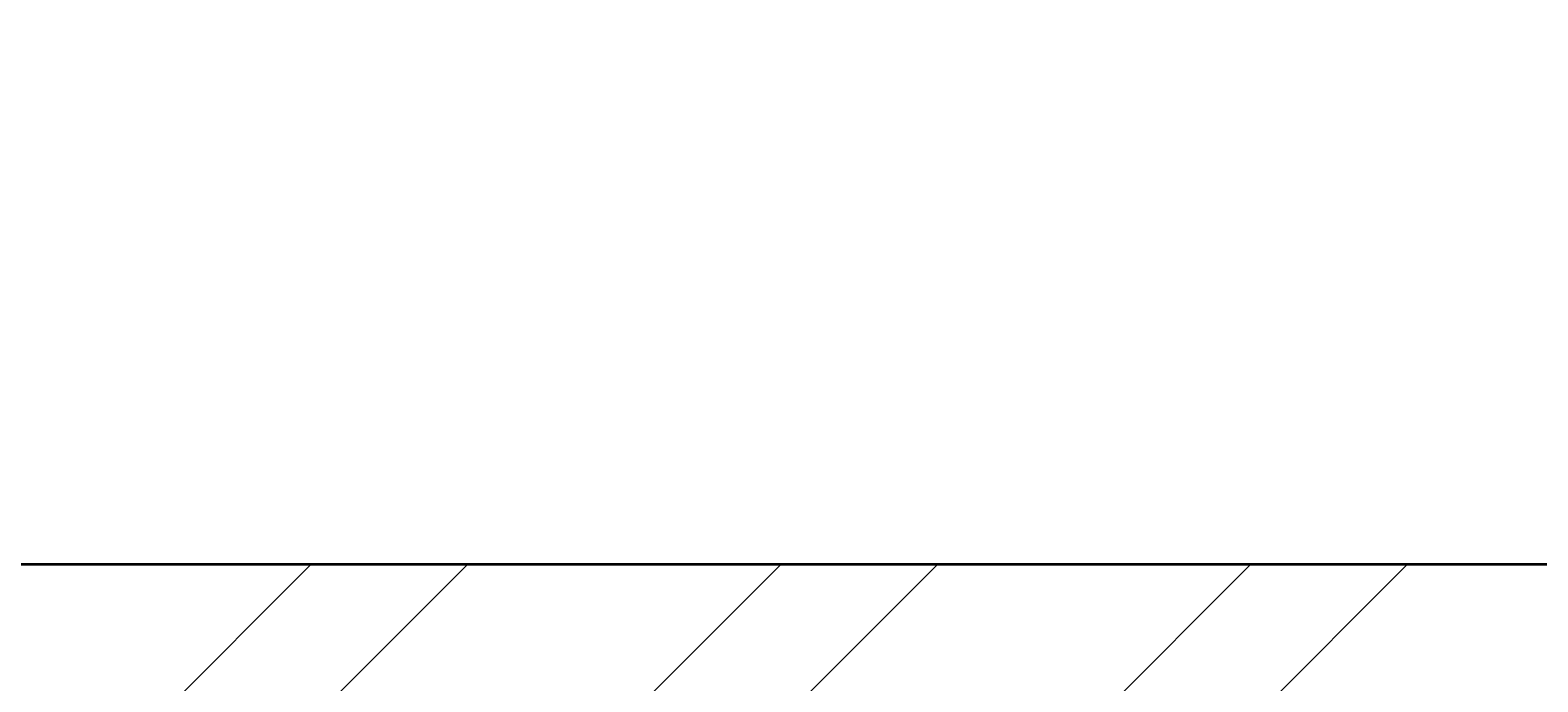
# Model space of a CAD drawing. Units: inches. Extents: x 1962 to 2771, y 1245 to 2660.
# Tile 51 of 114: x 2160 to 2204, y 2030 to 2049. Entities that reach past the tile are written whole.
import ezdxf

# ---------------------------------------------------------------- set-up
doc = ezdxf.new("R2010")
doc.units = ezdxf.units.IN
for name, color, linetype, lineweight in [('A-ANNO-DIMS', 2, 'Continuous', 18), ('A-WALL', 7, 'Continuous', 35), ('A-WALL-PATT', 252, 'Continuous', 13)]:
    doc.layers.add(name, color=color, linetype=linetype, lineweight=lineweight)
doc.styles.get("Standard").update_dxf_attribs({"font": 'arial.ttf'})
doc.dimstyles.get("Standard").update_dxf_attribs({"dimtxt": 0.18, "dimasz": 0.18, "dimexe": 0.18, "dimexo": 0.0625, "dimgap": 0.09, "dimtad": 0, "dimtih": 1, "dimtoh": 1, "dimdec": 4, "dimzin": 0, "dimdsep": 46, "dimtxsty": 'Standard', "dimcen": 0.09, "dimadec": 0, "dimazin": 0, "dimtfac": 1, "dimtdec": 4, "dimtofl": 0, "dimtmove": 0, "dimatfit": 3, "dimfxl": 1, "dimtolj": 1, "dimtzin": 0, "dimarcsym": 0})

# ---------------------------------------------------------------- blocks, each defined once
blk = doc.blocks.new('*D40')
at = {"layer": 'A-ANNO-DIMS', "color": 0, "lineweight": -2, "transparency": 16777216}
for p, q in [((2072.02, 2033.906), (2072.02, 2583.474)), ((2072.2, 2583.294), (2366.02, 2583.294)), ((2660.627, 2583.294), (2366.808, 2583.294)), ((2660.807, 2524.406), (2660.807, 2583.474))]:
    blk.add_line(p, q, dxfattribs=at)
at = {"layer": 'A-ANNO-DIMS', "color": 0, "transparency": 16777216}
for points in [[(2072.2, 2583.324), (2072.2, 2583.264), (2072.02, 2583.294)], [(2660.627, 2583.324), (2660.627, 2583.264), (2660.807, 2583.294)]]:
    blk.add_solid(points, dxfattribs=at)
at = {"layer": 'Defpoints', "color": 0, "transparency": 16777216}
for p in [(2660.807, 2583.294), (2660.807, 2524.344), (2072.02, 2033.844)]:
    blk.add_point(p, dxfattribs=at)
at = {"layer": 'A-ANNO-DIMS', "color": 0, "transparency": 16777216, "insert": (2366.414, 2583.294), "char_height": 0.18, "attachment_point": 5}
blk.add_mtext('\\A1;588.8', dxfattribs=at)

msp = doc.modelspace()

# ---------------------------------------------------------------- hatches: boundary and pattern name
at = {"layer": 'A-WALL-PATT'}
h = msp.add_hatch(dxfattribs=at)
h.set_pattern_fill('ANSI32', color=256)
h.paths.add_polyline_path([(2090.8074, 2467.3437), (2141.6481, 2467.3437), (2141.6481, 2469.5937), (2141.6481, 2471.8437), (2086.3074, 2471.8437), (2086.3074, 2422.5333), (2090.8074, 2422.5333)])
h.paths.add_polyline_path([(2282.7664, 2471.8437), (2204.8982, 2471.8437), (2204.8982, 2467.3437), (2234.8074, 2467.3437), (2234.8074, 2311.3437), (2228.7492, 2311.3437), (2228.7492, 2306.8437), (2234.8074, 2306.8437), (2331.9227, 2306.8437), (2331.9227, 2309.0937), (2331.9227, 2311.3437), (2239.3074, 2311.3437), (2239.3074, 2467.3437), (2282.7664, 2467.3437), (2282.7664, 2469.5937)])
h.paths.add_polyline_path([(2471.4531, 2519.8437), (2552.011, 2519.8437), (2564.3996, 2519.8437), (2564.3996, 2511.1389), (2568.8996, 2511.1389), (2568.8996, 2524.3437), (2466.9531, 2524.3437), (2466.9531, 2471.8437), (2450.0749, 2471.8437), (2446.4672, 2471.8437), (2446.4672, 2467.3437), (2450.0749, 2467.3437), (2475.9988, 2467.3437), (2475.9988, 2469.5937), (2475.9988, 2471.8437), (2471.4531, 2471.8437)])
h.paths.add_polyline_path([(2575.2231, 2469.5937), (2575.2231, 2471.8437), (2568.8996, 2471.8437), (2568.8996, 2487.1389), (2564.3996, 2487.1389), (2564.3996, 2471.8437), (2556.511, 2471.8437), (2499.2904, 2471.8437), (2499.2904, 2467.3437), (2507.8074, 2467.3437), (2507.8074, 2311.3437), (2414.863, 2311.3437), (2414.863, 2306.8437), (2512.3074, 2306.8437), (2517.0114, 2306.8437), (2517.0114, 2309.0937), (2517.0114, 2311.3437), (2512.3074, 2311.3437), (2512.3074, 2467.3437), (2575.2231, 2467.3437)])
h.paths.add_polyline_path([(2660.8074, 2471.8437), (2600.9602, 2471.8437), (2600.9602, 2467.3437), (2656.3074, 2467.3437), (2656.3074, 2432.5704), (2660.8074, 2432.5704)])
h.paths.add_polyline_path([(2660.8074, 2372.5704), (2656.3074, 2372.5704), (2656.3074, 2311.3437), (2600.276, 2311.3437), (2600.276, 2309.0937), (2600.276, 2306.8437), (2656.3074, 2306.8437), (2656.3074, 2296.2593), (2660.8074, 2296.2593)])
h.paths.add_polyline_path([(2572.3074, 2306.8437), (2577.1385, 2306.8437), (2577.1385, 2311.3437), (2551.082, 2311.3437), (2551.082, 2306.8437), (2567.8074, 2306.8437), (2567.8074, 2258.8437), (2540.0574, 2258.8437), (2540.0574, 2256.5937), (2540.0574, 2254.3437), (2567.8074, 2254.3437), (2656.3074, 2254.3437), (2656.3074, 2236.9085), (2660.8074, 2236.9085), (2660.8074, 2272.2593), (2656.3074, 2272.2593), (2656.3074, 2258.8437), (2572.3074, 2258.8437)])
h.paths.add_polyline_path([(2512.3074, 2254.3437), (2518.8716, 2254.3437), (2518.8716, 2256.5937), (2518.8716, 2258.8437), (2507.8074, 2258.8437), (2507.8074, 2177.8437), (2567.8074, 2177.8437), (2567.8074, 2172.9628), (2572.3074, 2172.9628), (2572.3074, 2177.8437), (2656.3074, 2177.8437), (2656.3074, 2166.4846), (2660.8074, 2166.4846), (2660.8074, 2200.9085), (2656.3074, 2200.9085), (2656.3074, 2182.3437), (2512.3074, 2182.3437)])
h.paths.add_polyline_path([(2656.3074, 2129.8437), (2572.3074, 2129.8437), (2572.3074, 2150.3044), (2570.0574, 2150.3044), (2567.8074, 2150.3044), (2567.8074, 2129.8437), (2507.8074, 2129.8437), (2507.8074, 2116.3027), (2510.0574, 2116.3027), (2512.3074, 2116.3027), (2512.3074, 2125.3437), (2567.8074, 2125.3437), (2572.3074, 2125.3437), (2656.3074, 2125.3437)])
h.paths.add_polyline_path([(2090.8074, 2362.5333), (2086.3074, 2362.5333), (2086.3074, 2298.6242), (2090.8074, 2298.6242), (2090.8074, 2306.8437), (2174.8074, 2306.8437), (2174.8074, 2286.4178), (2179.3074, 2286.4178), (2179.3074, 2306.8437), (2192.8641, 2306.8437), (2192.8641, 2309.0937), (2192.8641, 2311.3437), (2090.8074, 2311.3437)])
h.paths.add_polyline_path([(2209.156, 2258.8437), (2179.3074, 2258.8437), (2179.3074, 2263.2236), (2177.0574, 2263.2236), (2174.8074, 2263.2236), (2174.8074, 2258.8437), (2090.8074, 2258.8437), (2090.8074, 2274.6242), (2086.3074, 2274.6242), (2086.3074, 2238.2967), (2088.5574, 2238.2967), (2090.8074, 2238.2967), (2090.8074, 2254.3437), (2209.156, 2254.3437)])
h.paths.add_polyline_path([(2090.8074, 2177.8437), (2234.8074, 2177.8437), (2234.8074, 2173.1428), (2239.3074, 2173.1428), (2239.3074, 2258.8437), (2230.8442, 2258.8437), (2230.8442, 2256.5937), (2230.8442, 2254.3437), (2234.8074, 2254.3437), (2234.8074, 2182.3437), (2090.8074, 2182.3437), (2090.8074, 2202.2967), (2086.3074, 2202.2967), (2086.3074, 2140.0389), (2090.8074, 2140.0389)])
h.paths.add_polyline_path([(2090.8074, 2080.0389), (2086.3074, 2080.0389), (2086.3074, 2033.8437), (2090.8074, 2033.8437)], flags=17)
h.paths.add_polyline_path([(2244.9405, 2033.8437), (2239.3074, 2033.8437), (2239.3074, 2142.0665), (2237.2592, 2142.0665), (2234.8074, 2142.0665), (2234.8074, 2033.8437), (2090.8074, 2033.8437), (2076.5204, 2033.8437), (2072.0204, 2033.8437), (2072.0204, 2000.4493), (2076.5204, 2000.4493), (2076.5204, 2029.3437), (2090.8074, 2029.3437), (2244.9405, 2029.3437), (2244.9405, 2031.5937)])
h.paths.add_polyline_path([(2234.8074, 1933.3437), (2076.5204, 1933.3437), (2076.5204, 1952.4493), (2074.2704, 1952.4493), (2072.0204, 1952.4493), (2072.0204, 1933.3437), (2072.0204, 1928.8437), (2234.8074, 1928.8437)])
h.paths.add_polyline_path([(2090.8074, 1928.8437), (2086.3074, 1928.8437), (2086.3074, 1906.5013), (2090.8074, 1906.5013)])
h.paths.add_polyline_path([(2090.8074, 1846.5013), (2086.3074, 1846.5013), (2086.3074, 1769.9917), (2088.5574, 1769.9917), (2090.8074, 1769.9917), (2090.8074, 1780.3437), (2234.8074, 1780.3437), (2234.8074, 1708.3437), (2230.3764, 1708.3437), (2230.3764, 1703.8437), (2239.3074, 1703.8437), (2239.3074, 1792.6669), (2237.0574, 1792.6669), (2234.8074, 1792.6669), (2234.8074, 1784.8437), (2090.8074, 1784.8437)])
h.paths.add_polyline_path([(2239.3074, 1928.8437), (2244.9405, 1928.8437), (2244.9405, 1931.0937), (2244.9405, 1933.3437), (2234.8074, 1933.3437), (2234.8074, 1928.8437), (2234.8074, 1825.5949), (2239.3074, 1825.5949)])
h.paths.add_polyline_path([(2148.0425, 1649.0937), (2148.0425, 1651.3437), (2090.8074, 1651.3437), (2090.8074, 1646.8437), (2148.0425, 1646.8437)], flags=0)
h.paths.add_polyline_path([(2207.5601, 1708.3437), (2090.8074, 1708.3437), (2090.8074, 1703.8437), (2174.8074, 1703.8437), (2174.8074, 1651.3437), (2170.4457, 1651.3437), (2170.4457, 1646.8437), (2195.9924, 1646.8437), (2195.9924, 1649.0937), (2195.9924, 1651.3437), (2179.3074, 1651.3437), (2179.3074, 1703.8437), (2207.5601, 1703.8437), (2207.5601, 1706.0937)])
h.paths.add_polyline_path([(2090.8074, 1733.9917), (2086.3074, 1733.9917), (2086.3074, 1696.1032), (2088.5574, 1696.1032), (2090.8074, 1696.1032)])
h.paths.add_polyline_path([(2090.8074, 1672.1032), (2086.3074, 1672.1032), (2086.3074, 1600.3335), (2090.8074, 1600.3335)])
h.paths.add_polyline_path([(2090.8074, 1540.3335), (2086.3074, 1540.3335), (2086.3074, 1486.3437), (2139.6766, 1486.3437), (2139.6766, 1490.8437), (2090.8074, 1490.8437)])
h.paths.add_polyline_path([(2302.3876, 1490.8437), (2239.3074, 1490.8437), (2239.3074, 1646.8437), (2335.9994, 1646.8437), (2335.9994, 1651.3437), (2229.884, 1651.3437), (2229.884, 1646.8437), (2234.8074, 1646.8437), (2234.8074, 1490.8437), (2202.7103, 1490.8437), (2202.7103, 1488.5937), (2202.7103, 1486.3437), (2275.0699, 1486.3437), (2275.0699, 1475.772), (2279.5699, 1475.772), (2279.5699, 1486.3437), (2302.3876, 1486.3437)])
h.paths.add_polyline_path([(2279.5699, 1451.772), (2275.0699, 1451.772), (2275.0699, 1438.3437), (2174.8074, 1438.3437), (2174.8074, 1486.3437), (2179.7922, 1486.3437), (2179.7922, 1490.8437), (2163.3585, 1490.8437), (2163.3585, 1488.5937), (2163.3585, 1486.3437), (2170.3074, 1486.3437), (2170.3074, 1433.8437), (2279.5699, 1433.8437)])
h.paths.add_polyline_path([(2427.2363, 1490.8437), (2375.8074, 1490.8437), (2375.8074, 1646.8437), (2381.6401, 1646.8437), (2381.6401, 1651.3437), (2365.887, 1651.3437), (2365.887, 1649.0937), (2365.887, 1646.8437), (2371.3074, 1646.8437), (2371.3074, 1490.8437), (2327.5627, 1490.8437), (2327.5627, 1488.5937), (2327.5627, 1486.3437), (2371.3074, 1486.3437), (2371.3074, 1433.8437), (2375.8074, 1433.8437), (2375.8074, 1486.3437), (2427.2363, 1486.3437)])
h.paths.add_polyline_path([(2512.3074, 1646.8437), (2519.4351, 1646.8437), (2519.4351, 1649.0937), (2519.4351, 1651.3437), (2507.8074, 1651.3437), (2416.0063, 1651.3437), (2416.0063, 1649.0937), (2416.0063, 1646.8437), (2507.8074, 1646.8437), (2507.8074, 1490.8437), (2497.0532, 1490.8437), (2497.0532, 1488.5937), (2497.0532, 1486.3437), (2574.9344, 1486.3437), (2574.9344, 1476.0181), (2579.4344, 1476.0181), (2579.4344, 1486.3437), (2584.4872, 1486.3437), (2584.3074, 1490.8437), (2512.3074, 1490.8437)])
h.paths.add_polyline_path([(2470.5091, 1486.3437), (2473.9767, 1486.3437), (2473.9767, 1490.8437), (2449.6605, 1490.8437), (2449.6605, 1488.5937), (2449.6605, 1486.3437), (2466.0091, 1486.3437), (2466.0091, 1433.8437), (2470.5091, 1433.8437), (2579.4344, 1433.8437), (2579.4344, 1452.0181), (2574.9344, 1452.0181), (2574.9344, 1438.3437), (2554.5091, 1438.3437), (2470.5091, 1438.3437)])
h.paths.add_polyline_path([(2656.3074, 1490.8437), (2611.86, 1490.8437), (2611.86, 1486.3437), (2656.3074, 1486.3437)])
h.paths.add_polyline_path([(2660.8074, 1532.7007), (2658.5574, 1532.7007), (2656.3074, 1532.7007), (2656.3074, 1486.3437), (2660.8074, 1486.3437)])
h.paths.add_polyline_path([(2660.8074, 1664.9663), (2656.3074, 1664.9663), (2656.3074, 1651.3437), (2602.2313, 1651.3437), (2602.2313, 1646.8437), (2656.3074, 1646.8437), (2656.3074, 1592.7007), (2660.8074, 1592.7007)])
h.paths.add_polyline_path([(2660.8074, 1724.5221), (2656.3074, 1724.5221), (2656.3074, 1703.8437), (2542.4725, 1703.8437), (2542.4725, 1699.3437), (2567.8074, 1699.3437), (2567.8074, 1651.3437), (2552.7766, 1651.3437), (2552.7766, 1649.0937), (2552.7766, 1646.8437), (2577.2878, 1646.8437), (2577.2878, 1649.0937), (2577.2878, 1651.3437), (2572.3074, 1651.3437), (2572.3074, 1699.3437), (2656.3074, 1699.3437), (2656.3074, 1688.9663), (2660.8074, 1688.9663)])
h.paths.add_polyline_path([(2660.8074, 1880.6524), (2656.3074, 1880.6524), (2656.3074, 1832.8437), (2512.3074, 1832.8437), (2512.3074, 1837.8959), (2507.8074, 1837.8959), (2507.8074, 1828.3437), (2567.8074, 1828.3437), (2567.8074, 1804.3437), (2572.3074, 1804.3437), (2572.3074, 1828.3437), (2656.3074, 1828.3437), (2656.3074, 1818.6778), (2660.8074, 1818.6778)])
h.paths.add_polyline_path([(2660.8074, 1794.6778), (2656.3074, 1794.6778), (2656.3074, 1780.3437), (2572.3074, 1780.3437), (2572.3074, 1783.0303), (2570.0574, 1783.0303), (2567.8074, 1783.0303), (2567.8074, 1780.3437), (2507.8074, 1780.3437), (2507.8074, 1699.3437), (2517.8858, 1699.3437), (2517.8858, 1701.5937), (2517.8858, 1703.8437), (2512.3074, 1703.8437), (2512.3074, 1775.8437), (2656.3074, 1775.8437), (2656.3074, 1760.5221), (2660.8074, 1760.5221)])
h.paths.add_polyline_path([(2660.8074, 1981.3437), (2660.8074, 2020.2808), (2658.5574, 2020.2808), (2656.3074, 2020.2808), (2656.3074, 1981.3437), (2512.3074, 1981.3437), (2512.3074, 2086.6996), (2507.8074, 2086.6996), (2507.8074, 1981.3437), (2375.8074, 1981.3437), (2375.8074, 1986.8505), (2373.5574, 1986.8505), (2371.3074, 1986.8505), (2371.3074, 1973.2607), (2375.8074, 1973.2607), (2375.8074, 1976.8437), (2507.8074, 1976.8437), (2507.8074, 1865.4281), (2510.0574, 1865.4281), (2512.3074, 1865.4281), (2512.3074, 1976.8437), (2660.8074, 1976.8437)])
h.paths.add_polyline_path([(2375.8074, 1940.297), (2373.5574, 1940.297), (2371.3074, 1940.297), (2371.3074, 1933.3437), (2278.4434, 1933.3437), (2278.4434, 1928.8437), (2371.3074, 1928.8437), (2371.3074, 1651.3437), (2375.8074, 1651.3437)])
h.paths.add_polyline_path([(2660.8074, 1976.8437), (2656.3074, 1976.8437), (2656.3074, 1940.6524), (2660.8074, 1940.6524)], flags=17)
h.paths.add_polyline_path([(2660.8074, 2142.4846), (2656.3074, 2142.4846), (2656.3074, 2080.2808), (2660.8074, 2080.2808)])
h.paths.add_polyline_path([(2381.4189, 2311.3437), (2375.8074, 2311.3437), (2375.8074, 2467.3437), (2424.7242, 2467.3437), (2424.7242, 2469.5937), (2424.7242, 2471.8437), (2375.8074, 2471.8437), (2375.8074, 2524.3437), (2371.3074, 2524.3437), (2371.3074, 2471.8437), (2307.2097, 2471.8437), (2307.2097, 2467.3437), (2371.3074, 2467.3437), (2371.3074, 2311.3437), (2366.8901, 2311.3437), (2366.8901, 2306.8437), (2371.3074, 2306.8437), (2371.3074, 2033.8437), (2279.6589, 2033.8437), (2279.6589, 2029.3437), (2371.3074, 2029.3437), (2371.3074, 2014.2598), (2375.8074, 2014.2598), (2375.8074, 2306.8437), (2381.4189, 2306.8437)])
h.paths.add_polyline_path([(2263.3074, 2524.3437), (2170.3074, 2524.3437), (2170.3074, 2519.8437), (2170.3074, 2471.8437), (2165.0312, 2471.8437), (2165.0312, 2467.3437), (2179.6721, 2467.3437), (2179.6721, 2469.5161), (2179.6721, 2471.8437), (2174.8074, 2471.8437), (2174.8074, 2519.8437), (2258.8074, 2519.8437), (2258.8074, 2511.6436), (2263.3074, 2511.6436)])
h.paths.add_polyline_path([(2245.0232, 1361.4123), (2492.9468, 1361.4123), (2492.9468, 1398.505), (2245.0232, 1398.505)], flags=9)
h.paths.add_polyline_path([(2388.1434, 2086.6936), (2425.0704, 2086.6936), (2425.0704, 2105.3509), (2388.1434, 2105.3509)], flags=9)
h.paths.add_polyline_path([(2404.922, 2242.6744), (2445.7337, 2242.6744), (2445.7337, 2261.3318), (2404.922, 2261.3318)], flags=9)
h.paths.add_polyline_path([(2269.4107, 2156.7935), (2306.3378, 2156.7935), (2306.3378, 2175.4508), (2269.4107, 2175.4508)], flags=9)
h.paths.add_polyline_path([(2269.3277, 2233.4343), (2306.2547, 2233.4343), (2306.2547, 2252.0917), (2269.3277, 2252.0917)], flags=9)
h.paths.add_polyline_path([(2431.6052, 2320.6922), (2470.4456, 2320.6922), (2470.4456, 2339.3495), (2431.6052, 2339.3495)], flags=25)
h.paths.add_polyline_path([(2249.6902, 2315.7608), (2288.5306, 2315.7608), (2288.5306, 2334.4182), (2249.6902, 2334.4182)], flags=25)
h.paths.add_polyline_path([(2096.9301, 2314.3181), (2135.7704, 2314.3181), (2135.7704, 2332.9755), (2096.9301, 2332.9755)], flags=25)
h.paths.add_polyline_path([(2134.3475, 2285.7089), (2161.4655, 2285.7089), (2161.4655, 2304.3662), (2134.3475, 2304.3662)], flags=9)
h.paths.add_polyline_path([(2126.5155, 2209.4076), (2159.9227, 2209.4076), (2159.9227, 2228.065), (2126.5155, 2228.065)], flags=25)
h.paths.add_polyline_path([(2110.5753, 2141.5299), (2149.4157, 2141.5299), (2149.4157, 2160.1872), (2110.5753, 2160.1872)], flags=25)
h.paths.add_polyline_path([(2249.8618, 1968.3317), (2286.3966, 1968.3317), (2286.3966, 1986.989), (2249.8618, 1986.989)], flags=9)
h.paths.add_polyline_path([(2395.9507, 1777.0051), (2436.7624, 1777.0051), (2436.7624, 1795.6625), (2395.9507, 1795.6625)], flags=9)
h.paths.add_polyline_path([(2398.5259, 1888.5651), (2435.0062, 1888.5651), (2435.0062, 1907.2224), (2398.5259, 1907.2224)], flags=25)
h.paths.add_polyline_path([(2259.3506, 1728.3559), (2296.2776, 1728.3559), (2296.2776, 1747.0132), (2259.3506, 1747.0132)], flags=9)
h.paths.add_polyline_path([(2271.3698, 1845.268), (2308.2968, 1845.268), (2308.2968, 1863.9253), (2271.3698, 1863.9253)], flags=9)
h.paths.add_polyline_path([(2120.9355, 1786.3027), (2159.7759, 1786.3027), (2159.7759, 1804.9601), (2120.9355, 1804.9601)], flags=25)
h.paths.add_polyline_path([(2121.3164, 1732.1043), (2154.7236, 1732.1043), (2154.7236, 1750.7616), (2121.3164, 1750.7616)], flags=25)
h.paths.add_polyline_path([(2118.3706, 1678.8997), (2147.5282, 1678.8997), (2147.5282, 1697.557), (2118.3706, 1697.557)], flags=25)
h.paths.add_polyline_path([(2385.9227, 1493.557), (2424.763, 1493.557), (2424.763, 1512.2143), (2385.9227, 1512.2143)], flags=25)
h.paths.add_polyline_path([(2248.7058, 1500.0256), (2287.5462, 1500.0256), (2287.5462, 1518.6829), (2248.7058, 1518.6829)], flags=25)
h.paths.add_polyline_path([(2104.1669, 1617.3771), (2143.0073, 1617.3771), (2143.0073, 1636.0344), (2104.1669, 1636.0344)], flags=9)
h.paths.add_polyline_path([(2096.0714, 1447.8824), (2137.3845, 1447.8824), (2137.3845, 1458.1859), (2096.0714, 1458.1859)], flags=9)
h.paths.add_polyline_path([(2180.6114, 1440.325), (2209.7689, 1440.325), (2209.7689, 1458.9823), (2180.6114, 1458.9823)], flags=25)
h.paths.add_polyline_path([(2316.1698, 1447.9637), (2357.4829, 1447.9637), (2357.4829, 1458.2673), (2316.1698, 1458.2673)], flags=9)
h.paths.add_polyline_path([(2397.6187, 1447.9637), (2438.9318, 1447.9637), (2438.9318, 1458.2673), (2397.6187, 1458.2673)], flags=9)
h.paths.add_polyline_path([(2473.0778, 1439.5953), (2502.2354, 1439.5953), (2502.2354, 1458.2527), (2473.0778, 1458.2527)], flags=25)
h.paths.add_polyline_path([(2589.7027, 1447.8819), (2631.0158, 1447.8819), (2631.0158, 1458.1855), (2589.7027, 1458.1855)], flags=9)
h.paths.add_polyline_path([(2522.4009, 1497.5285), (2561.2413, 1497.5285), (2561.2413, 1516.1859), (2522.4009, 1516.1859)], flags=25)
h.paths.add_polyline_path([(2579.6565, 1671.3482), (2608.8141, 1671.3482), (2608.8141, 1690.0056), (2579.6565, 1690.0056)], flags=25)
h.paths.add_polyline_path([(2544.7038, 1725.5064), (2578.1111, 1725.5064), (2578.1111, 1744.1637), (2544.7038, 1744.1637)], flags=25)
h.paths.add_polyline_path([(2578.1191, 1807.472), (2607.2766, 1807.472), (2607.2766, 1826.1293), (2578.1191, 1826.1293)], flags=25)
h.paths.add_polyline_path([(2595.0614, 1835.1839), (2633.9018, 1835.1839), (2633.9018, 1853.8413), (2595.0614, 1853.8413)], flags=25)
h.paths.add_polyline_path([(2567.0097, 2097.7035), (2605.8501, 2097.7035), (2605.8501, 2116.3609), (2567.0097, 2116.3609)], flags=9)
h.paths.add_polyline_path([(2586.644, 2134.6454), (2615.8015, 2134.6454), (2615.8015, 2153.3027), (2586.644, 2153.3027)], flags=9)
h.paths.add_polyline_path([(2544.6185, 2212.6783), (2578.0258, 2212.6783), (2578.0258, 2231.3356), (2544.6185, 2231.3356)], flags=25)
h.paths.add_polyline_path([(2577.0273, 2256.9023), (2606.1849, 2256.9023), (2606.1849, 2275.5597), (2577.0273, 2275.5597)], flags=24)
h.paths.add_polyline_path([(2605.2683, 2315.2821), (2644.1087, 2315.2821), (2644.1087, 2333.9395), (2605.2683, 2333.9395)], flags=25)
h.paths.add_polyline_path([(2583.1244, 2496.1815), (2624.4375, 2496.1815), (2624.4375, 2506.4851), (2583.1244, 2506.4851)], flags=9)
h.paths.add_polyline_path([(2474.761, 2497.0823), (2503.9185, 2497.0823), (2503.9185, 2515.7397), (2474.761, 2515.7397)], flags=25)
h.paths.add_polyline_path([(2387.5787, 2494.2563), (2428.902, 2494.2563), (2428.902, 2504.5598), (2387.5787, 2504.5598)], flags=9)
h.paths.add_polyline_path([(2300.1657, 2500.1564), (2341.4788, 2500.1564), (2341.4788, 2510.46), (2300.1657, 2510.46)], flags=25)
h.paths.add_polyline_path([(2176.8589, 2497.5843), (2206.0165, 2497.5843), (2206.0165, 2516.2416), (2176.8589, 2516.2416)], flags=25)
h.paths.add_polyline_path([(2097.4668, 2494.9762), (2138.7799, 2494.9762), (2138.7799, 2505.2798), (2097.4668, 2505.2798)], flags=9)

# ---------------------------------------------------------------- linework, layer by layer
at = {"layer": 'A-WALL'}
msp.add_line((2090.8074, 2033.8437), (2234.8074, 2033.8437), dxfattribs=at)

# ---------------------------------------------------------------- dimensions: what is measured, and where the dimension line sits
at = {"layer": 'A-ANNO-DIMS'}
dim = msp.add_linear_dim(base=(2660.8074, 2583.2937), p1=(2072.0204, 2033.8437), p2=(2660.8074, 2524.3437), dimstyle='Standard', override={"dimdec": 1, "dimlfac": 1, "dimrnd": 0, "dimzin": 0, "dimdsep": 46, "dimlunit": 2}, dxfattribs=at)
dim.commit()
dim.dimension.update_dxf_attribs({"geometry": '*D40', "text_midpoint": (2366.4139, 2583.2937)})

doc.saveas('drawing.dxf')
